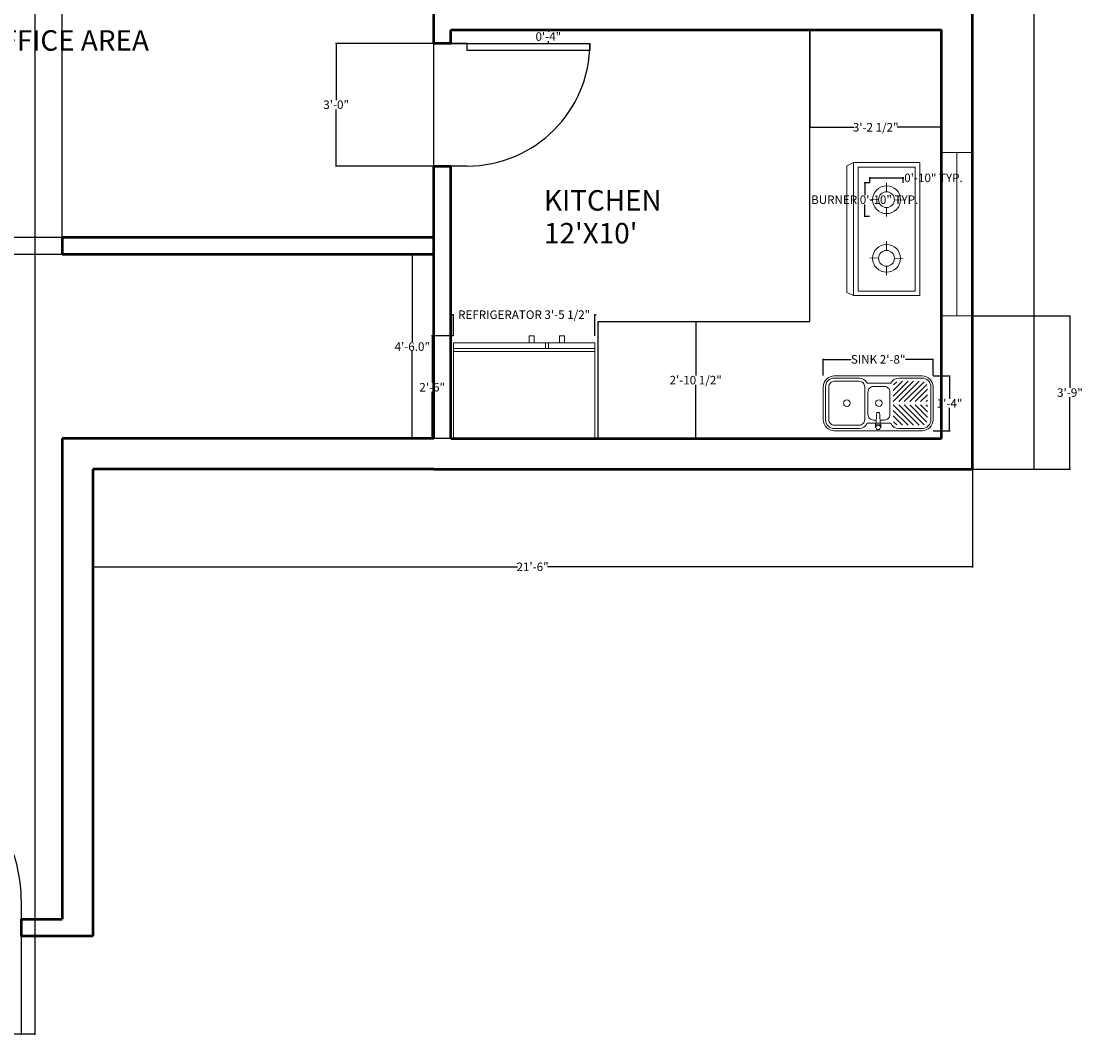
# Model space of a CAD drawing. Units: inches. Extents: x 9441 to 10027, y 18319 to 18830.
# Tile 3 of 4: x 9716 to 10027, y 18319 to 18618. Entities that reach past the tile are written whole.
import ezdxf

# ---------------------------------------------------------------- set-up
doc = ezdxf.new("R2010")
doc.units = ezdxf.units.IN
doc.header["$MEASUREMENT"] = 0
for name, color, linetype, lineweight in [('A-ANNO-DIMS', 2, 'Continuous', 18), ('A-AREA-IDEN', 7, 'Continuous', 25), ('A-DOOR', 3, 'Continuous', 25), ('A-FLOR-CABT', 9, 'Continuous', 25), ('A-FLOR-FIXT', 9, 'Continuous', 18), ('A-GLAZ', 4, 'Continuous', 18), ('A-WALL', 7, 'Continuous', 50), ('equipments', 8, 'Continuous', 20)]:
    doc.layers.add(name, color=color, linetype=linetype, lineweight=lineweight)
doc.styles.get("Standard").update_dxf_attribs({"font": 'arial.ttf'})
doc.dimstyles.get("Standard").update_dxf_attribs({"dimtxt": 2.5, "dimasz": 0.18, "dimexe": 0.18, "dimexo": 0.0625, "dimgap": 0.09, "dimtad": 0, "dimtih": 1, "dimtoh": 1, "dimdec": 1, "dimzin": 0, "dimdsep": 46, "dimlunit": 3, "dimtxsty": 'Standard', "dimcen": 0.09, "dimadec": 0, "dimazin": 0, "dimtfac": 1, "dimtdec": 1, "dimtofl": 0, "dimtmove": 0, "dimatfit": 3, "dimfxl": 1, "dimtolj": 1, "dimtzin": 0, "dimarcsym": 0})

# ---------------------------------------------------------------- blocks, each defined once
blk = doc.blocks.new('*U2')
for p, q in [((0, 0), (0, -100)), ((750, 0), (750, -100))]:
    blk.add_line(p, q)
blk.add_lwpolyline([(0, 0), (0, 750), (43.75, 750), (43.75, 0)], close=True)
blk.add_arc((0, 0), 750, 0, 90)
blk = doc.blocks.new('*U4')
for p, q in [((0, 100), (0, 0)), ((900, 100), (900, 0)), ((0, 50), (900, 50))]:
    blk.add_line(p, q)
blk = doc.blocks.new('C12')
for p, q in [((-0.70131, -0.87335), (-0.70131, -0.00485)), ((0.58127, -0.00485), (-0.70131, -0.00485)), ((0.58127, -0.87335), (0.58127, -0.00485)), ((-0.70131, -0.79423), (0.58127, -0.79423)), ((-0.70131, -0.82077), (0.58127, -0.82077)), ((-0.27938, -0.87335), (-0.27938, -0.82077)), ((-0.25493, -0.87335), (-0.25493, -0.82077)), ((-0.70131, -0.87335), (0.58127, -0.87335)), ((-0.42655, -0.93628), (-0.42655, -0.8713)), ((-0.38018, -0.8713), (-0.38018, -0.93628)), ((-0.15115, -0.8713), (-0.15115, -0.93628)), ((-0.10477, -0.93628), (-0.10477, -0.8713)), ((-0.38018, -0.93628), (-0.42655, -0.93628)), ((-0.15115, -0.93628), (-0.10477, -0.93628))]:
    blk.add_line(p, q)
blk = doc.blocks.new('62438789')
at = {"xscale": 10, "zscale": 10}
blk.add_blockref('C12', (0.9326, -0.0075), dxfattribs=at)
blk = doc.blocks.new('REFRIG4')
at = {"xscale": 0.1, "zscale": 0.1}
blk.add_blockref('62438789', (-0.0332, 0.0123), dxfattribs=at)
blk = doc.blocks.new('SINK_KITCHEN2')
for p, q in [((13.7, -23.5), (32.2, -5)), ((13.7, -13.5), (22.2, -5)), ((13.7, -18.5), (27.2, -5)), ((14.06, -8.14), (16.84, -5.36)), ((18.7, -23.5), (37.2, -5)), ((23.7, -23.5), (41.85, -5.35)), ((28.7, -23.5), (44.46, -7.74)), ((1.2, -16.49), (-1.2, -16.49)), ((33.7, -23.5), (45, -12.2)), ((38.7, -23.5), (45, -17.2)), ((13.7, -26.5), (32.2, -45)), ((18.7, -26.5), (37.2, -45)), ((23.7, -26.5), (41.85, -44.65)), ((28.7, -26.5), (44.46, -42.26)), ((33.7, -26.5), (45, -37.8)), ((38.7, -26.5), (45, -32.8)), ((43.7, -23.5), (45, -22.2)), ((43.7, -26.5), (45, -27.8)), ((13.7, -31.5), (27.2, -45)), ((13.7, -36.5), (22.2, -45)), ((14.06, -41.86), (16.84, -44.64))]:
    blk.add_line(p, q)
at = {"flags": 128}
for points in [[(-40, -50, -0.414214), (-50, -40), (-50, -10, -0.414214), (-40, 0), (40, 0, -0.414214), (50, -10), (50, -40, -0.414214), (40, -50)], [(-40, -45, -0.414214), (-45, -40), (-45, -10, -0.414214), (-40, -5), (-17.3, -5, -0.414214), (-12.3, -10), (-12.3, -40, -0.414214), (-17.3, -45)]]:
    blk.add_lwpolyline(points, format="xyb", close=True, dxfattribs=at)
for points in [[(2.5, -6.75), (11.39, -6.75, -0.296358), (18.7, -2), (40, -2, -0.414214), (48, -10), (48, -40, -0.414214), (40, -48), (18.7, -48, -0.296358), (11.39, -43.25), (-9.99, -43.25, -0.296358), (-17.3, -48), (-40, -48, -0.414214), (-48, -40), (-48, -10, -0.414214), (-40, -2), (-17.3, -2, -0.296358), (-9.99, -6.75), (-2.5, -6.75)], [(1.2, -16.49, 0.016708), (1.9, -6.98, 0.016708)], [(1.76, -9.75), (5.7, -9.75, -0.414214), (10.7, -14.75), (10.7, -35.25, -0.414214), (5.7, -40.25), (-4.3, -40.25, -0.414214), (-9.3, -35.25), (-9.3, -14.75, -0.414214), (-4.3, -9.75), (-1.76, -9.75)]]:
    blk.add_lwpolyline(points, format="xyb", dxfattribs=at)
blk.add_lwpolyline([(-2, -5.48), (2, -5.48), (2, -3), (2.5, -3), (2.5, -6.98), (-2.5, -6.98), (-2.5, -3), (-2, -3)], close=True)
for centre, radius in [((0, -3), 2), ((-28.65, -25), 3), ((0.7, -25), 3)]:
    blk.add_circle(centre, radius)
blk.add_arc((140.8, -1.2), 142.82, 182.31735, 186.14617)
blk = doc.blocks.new('*D14')
at = {"layer": 'A-ANNO-DIMS', "color": 0, "lineweight": -2, "transparency": 16777216}
for p, q in [((9836.83, 18549.93), (9830.42, 18549.93)), ((9830.6, 18549.75), (9830.6, 18524.29)), ((9830.6, 18496.11), (9830.6, 18521.56)), ((9836.83, 18495.93), (9830.42, 18495.93))]:
    blk.add_line(p, q, dxfattribs=at)
at = {"layer": 'A-ANNO-DIMS', "color": 0, "transparency": 16777216}
for points in [[(9830.57, 18549.75), (9830.63, 18549.75), (9830.6, 18549.93)], [(9830.57, 18496.11), (9830.63, 18496.11), (9830.6, 18495.93)]]:
    blk.add_solid(points, dxfattribs=at)
at = {"layer": 'Defpoints', "color": 0, "transparency": 16777216}
for p in [(9830.6, 18549.93), (9836.89, 18549.93), (9836.89, 18495.93)]:
    blk.add_point(p, dxfattribs=at)
at = {"layer": 'A-ANNO-DIMS', "color": 0, "transparency": 16777216, "insert": (9830.6, 18522.93), "char_height": 2.5, "attachment_point": 5}
blk.add_mtext('\\A1;4\'-6.0"', dxfattribs=at)
blk = doc.blocks.new('*D17')
at = {"layer": 'A-ANNO-DIMS', "color": 0, "lineweight": -2, "transparency": 16777216}
for p, q in [((9994.95, 18797.93), (10013.22, 18797.93)), ((10013.04, 18797.75), (10013.04, 18643.79)), ((10013.04, 18487.11), (10013.04, 18641.06)), ((9994.95, 18486.93), (10013.22, 18486.93))]:
    blk.add_line(p, q, dxfattribs=at)
at = {"layer": 'A-ANNO-DIMS', "color": 0, "transparency": 16777216}
for points in [[(10013.01, 18797.75), (10013.07, 18797.75), (10013.04, 18797.93)], [(10013.01, 18487.11), (10013.07, 18487.11), (10013.04, 18486.93)]]:
    blk.add_solid(points, dxfattribs=at)
at = {"layer": 'Defpoints', "color": 0, "transparency": 16777216}
for p in [(9994.89, 18797.93), (10013.04, 18797.93), (9994.89, 18486.93)]:
    blk.add_point(p, dxfattribs=at)
at = {"layer": 'A-ANNO-DIMS', "color": 0, "transparency": 16777216, "insert": (10013.04, 18642.43), "char_height": 2.5, "attachment_point": 5}
blk.add_mtext('\\A1;25\'-11.0"', dxfattribs=at)
blk = doc.blocks.new('WIN-FRAME-48x9')
for p, q in [((48, 9), (0, 9)), ((0, 9), (0, 0)), ((48, 0), (48, 9))]:
    blk.add_line(p, q)
blk = doc.blocks.new('COOKTOP-BURNER')
for p, q in [((4.94, 7.25), (4.95, 9.86)), ((2.61, 5), (0, 5.08)), ((7.25, 4.86), (9.85, 4.78)), ((4.92, 2.61), (4.9, 0))]:
    blk.add_line(p, q)
for radius in [4.08, 2.32]:
    blk.add_circle((4.93, 4.93), radius)
blk = doc.blocks.new('*D31')
at = {"layer": 'A-ANNO-DIMS', "color": 0, "lineweight": -2, "transparency": 16777216}
for p, q in [((9964.72, 18570.97), (9963.13, 18570.97)), ((9963.31, 18570.79), (9963.31, 18567.41)), ((9963.31, 18561.29), (9963.31, 18564.68)), ((9964.72, 18561.11), (9963.13, 18561.11))]:
    blk.add_line(p, q, dxfattribs=at)
at = {"layer": 'A-ANNO-DIMS', "color": 0, "transparency": 16777216}
for points in [[(9963.28, 18570.79), (9963.34, 18570.79), (9963.31, 18570.97)], [(9963.28, 18561.29), (9963.34, 18561.29), (9963.31, 18561.11)]]:
    blk.add_solid(points, dxfattribs=at)
at = {"layer": 'Defpoints', "color": 0, "transparency": 16777216}
for p in [(9963.31, 18570.97), (9964.79, 18570.97), (9964.79, 18561.11)]:
    blk.add_point(p, dxfattribs=at)
at = {"layer": 'A-ANNO-DIMS', "color": 0, "transparency": 16777216, "insert": (9963.31, 18566.04), "char_height": 2.5, "attachment_point": 5}
blk.add_mtext('\\A1;BURNER 0\'-10" TYP.', dxfattribs=at)
blk = doc.blocks.new('*D32')
at = {"layer": 'A-ANNO-DIMS', "color": 0, "lineweight": -2, "transparency": 16777216}
for p, q in [((9964.79, 18571.03), (9964.79, 18572.63)), ((9964.97, 18572.45), (9974.46, 18572.45)), ((9974.64, 18571.03), (9974.64, 18572.63)), ((9974.64, 18572.45), (9974.82, 18572.45))]:
    blk.add_line(p, q, dxfattribs=at)
at = {"layer": 'A-ANNO-DIMS', "color": 0, "transparency": 16777216}
for points in [[(9964.97, 18572.48), (9964.97, 18572.42), (9964.79, 18572.45)], [(9974.46, 18572.48), (9974.46, 18572.42), (9974.64, 18572.45)]]:
    blk.add_solid(points, dxfattribs=at)
at = {"layer": 'Defpoints', "color": 0, "transparency": 16777216}
for p in [(9974.64, 18572.45), (9964.79, 18570.97), (9974.64, 18570.97)]:
    blk.add_point(p, dxfattribs=at)
at = {"layer": 'A-ANNO-DIMS', "color": 0, "transparency": 16777216, "insert": (9983.5, 18572.45), "char_height": 2.5, "attachment_point": 5}
blk.add_mtext('\\A1;0\'-10" TYP.', dxfattribs=at)
blk = doc.blocks.new('*D33')
at = {"layer": 'A-ANNO-DIMS', "color": 0, "lineweight": -2, "transparency": 16777216}
for p, q in [((9842.49, 18532.3), (9842.31, 18532.3)), ((9842.67, 18526.13), (9842.67, 18532.48)), ((9884.18, 18526.13), (9884.18, 18532.48)), ((9884.36, 18532.3), (9884.54, 18532.3))]:
    blk.add_line(p, q, dxfattribs=at)
at = {"layer": 'A-ANNO-DIMS', "color": 0, "transparency": 16777216}
for points in [[(9842.49, 18532.33), (9842.49, 18532.27), (9842.67, 18532.3)], [(9884.36, 18532.33), (9884.36, 18532.27), (9884.18, 18532.3)]]:
    blk.add_solid(points, dxfattribs=at)
at = {"layer": 'Defpoints', "color": 0, "transparency": 16777216}
for p in [(9842.67, 18532.3), (9842.67, 18526.07), (9884.18, 18526.07)]:
    blk.add_point(p, dxfattribs=at)
at = {"layer": 'A-ANNO-DIMS', "color": 0, "transparency": 16777216, "insert": (9863.42, 18532.3), "char_height": 2.5, "attachment_point": 5}
blk.add_mtext('\\A1;REFRIGERATOR 3\'-5 1/2"', dxfattribs=at)
blk = doc.blocks.new('*D34')
at = {"layer": 'A-ANNO-DIMS', "color": 0, "lineweight": -2, "transparency": 16777216}
for p, q in [((9842.61, 18526.07), (9836.26, 18526.07)), ((9836.44, 18525.89), (9836.44, 18512.36)), ((9836.44, 18496.11), (9836.44, 18509.63)), ((9842.61, 18495.93), (9836.26, 18495.93))]:
    blk.add_line(p, q, dxfattribs=at)
at = {"layer": 'A-ANNO-DIMS', "color": 0, "transparency": 16777216}
for points in [[(9836.41, 18525.89), (9836.47, 18525.89), (9836.44, 18526.07)], [(9836.41, 18496.11), (9836.47, 18496.11), (9836.44, 18495.93)]]:
    blk.add_solid(points, dxfattribs=at)
at = {"layer": 'Defpoints', "color": 0, "transparency": 16777216}
for p in [(9842.67, 18526.07), (9836.44, 18495.93), (9842.67, 18495.93)]:
    blk.add_point(p, dxfattribs=at)
at = {"layer": 'A-ANNO-DIMS', "color": 0, "transparency": 16777216, "insert": (9836.44, 18511), "char_height": 2.5, "attachment_point": 5}
blk.add_mtext('\\A1;2\'-6"', dxfattribs=at)
blk = doc.blocks.new('*D35')
at = {"layer": 'A-ANNO-DIMS', "color": 0, "lineweight": -2, "transparency": 16777216}
for p, q in [((9951.17, 18514.41), (9951.17, 18519.36)), ((9951.35, 18519.18), (9959.3, 18519.18)), ((9983.19, 18519.18), (9975.24, 18519.18)), ((9983.37, 18514.41), (9983.37, 18519.36))]:
    blk.add_line(p, q, dxfattribs=at)
at = {"layer": 'A-ANNO-DIMS', "color": 0, "transparency": 16777216}
for points in [[(9951.35, 18519.21), (9951.35, 18519.15), (9951.17, 18519.18)], [(9983.19, 18519.21), (9983.19, 18519.15), (9983.37, 18519.18)]]:
    blk.add_solid(points, dxfattribs=at)
at = {"layer": 'Defpoints', "color": 0, "transparency": 16777216}
for p in [(9983.37, 18519.18), (9951.17, 18514.35), (9983.37, 18514.35)]:
    blk.add_point(p, dxfattribs=at)
at = {"layer": 'A-ANNO-DIMS', "color": 0, "transparency": 16777216, "insert": (9967.27, 18519.18), "char_height": 2.5, "attachment_point": 5}
blk.add_mtext('\\A1;SINK 2\'-8"', dxfattribs=at)
blk = doc.blocks.new('*D36')
at = {"layer": 'A-ANNO-DIMS', "color": 0, "lineweight": -2, "transparency": 16777216}
for p, q in [((9983.43, 18514.35), (9988.38, 18514.35)), ((9988.2, 18514.17), (9988.2, 18507.65)), ((9988.2, 18498.43), (9988.2, 18504.96)), ((9983.43, 18498.25), (9988.38, 18498.25))]:
    blk.add_line(p, q, dxfattribs=at)
at = {"layer": 'A-ANNO-DIMS', "color": 0, "transparency": 16777216}
for points in [[(9988.17, 18514.17), (9988.23, 18514.17), (9988.2, 18514.35)], [(9988.17, 18498.43), (9988.23, 18498.43), (9988.2, 18498.25)]]:
    blk.add_solid(points, dxfattribs=at)
at = {"layer": 'Defpoints', "color": 0, "transparency": 16777216}
for p in [(9983.37, 18514.35), (9983.37, 18498.25), (9988.2, 18498.25)]:
    blk.add_point(p, dxfattribs=at)
at = {"layer": 'A-ANNO-DIMS', "color": 0, "transparency": 16777216, "insert": (9988.2, 18506.3), "char_height": 2.5, "attachment_point": 5}
blk.add_mtext('\\A1;1\'-4"', dxfattribs=at)
blk = doc.blocks.new('*D37')
at = {"layer": 'A-ANNO-DIMS', "color": 0, "lineweight": -2, "transparency": 16777216}
for p, q in [((9736.89, 18486.86), (9736.89, 18458.12)), ((9994.89, 18486.86), (9994.89, 18458.12)), ((9737.07, 18458.3), (9861.49, 18458.3)), ((9994.71, 18458.3), (9870.3, 18458.3))]:
    blk.add_line(p, q, dxfattribs=at)
at = {"layer": 'A-ANNO-DIMS', "color": 0, "transparency": 16777216}
for points in [[(9737.07, 18458.33), (9737.07, 18458.27), (9736.89, 18458.3)], [(9994.71, 18458.33), (9994.71, 18458.27), (9994.89, 18458.3)]]:
    blk.add_solid(points, dxfattribs=at)
at = {"layer": 'Defpoints', "color": 0, "transparency": 16777216}
for p in [(9736.89, 18486.93), (9994.89, 18486.93), (9736.89, 18458.3)]:
    blk.add_point(p, dxfattribs=at)
at = {"layer": 'A-ANNO-DIMS', "color": 0, "transparency": 16777216, "insert": (9865.89, 18458.3), "char_height": 2.5, "attachment_point": 5}
blk.add_mtext('\\A1;21\'-6"', dxfattribs=at)
blk = doc.blocks.new('*D40')
at = {"layer": 'A-ANNO-DIMS', "color": 0, "lineweight": -2, "transparency": 16777216}
for p, q in [((9673.89, 18349.86), (9673.89, 18320.95)), ((9715.89, 18349.86), (9715.89, 18320.95)), ((9674.07, 18321.13), (9691.48, 18321.13)), ((9715.71, 18321.13), (9698.3, 18321.13))]:
    blk.add_line(p, q, dxfattribs=at)
at = {"layer": 'A-ANNO-DIMS', "color": 0, "transparency": 16777216}
for points in [[(9674.07, 18321.16), (9674.07, 18321.1), (9673.89, 18321.13)], [(9715.71, 18321.16), (9715.71, 18321.1), (9715.89, 18321.13)]]:
    blk.add_solid(points, dxfattribs=at)
at = {"layer": 'Defpoints', "color": 0, "transparency": 16777216}
for p in [(9673.89, 18349.93), (9715.89, 18349.93), (9715.89, 18321.13)]:
    blk.add_point(p, dxfattribs=at)
at = {"layer": 'A-ANNO-DIMS', "color": 0, "transparency": 16777216, "insert": (9694.89, 18321.13), "char_height": 2.5, "attachment_point": 5}
blk.add_mtext('\\A1;3\'-6"', dxfattribs=at)
blk = doc.blocks.new('*D46')
at = {"layer": 'A-ANNO-DIMS', "color": 0, "lineweight": -2, "transparency": 16777216}
for p, q in [((9994.95, 18531.93), (10023.7, 18531.93)), ((10023.52, 18531.75), (10023.52, 18510.79)), ((10023.52, 18487.11), (10023.52, 18508.06)), ((9994.95, 18486.93), (10023.7, 18486.93))]:
    blk.add_line(p, q, dxfattribs=at)
at = {"layer": 'A-ANNO-DIMS', "color": 0, "transparency": 16777216}
for points in [[(10023.49, 18531.75), (10023.55, 18531.75), (10023.52, 18531.93)], [(10023.49, 18487.11), (10023.55, 18487.11), (10023.52, 18486.93)]]:
    blk.add_solid(points, dxfattribs=at)
at = {"layer": 'Defpoints', "color": 0, "transparency": 16777216}
for p in [(9994.89, 18531.93), (10023.52, 18531.93), (9994.89, 18486.93)]:
    blk.add_point(p, dxfattribs=at)
at = {"layer": 'A-ANNO-DIMS', "color": 0, "transparency": 16777216, "insert": (10023.52, 18509.43), "char_height": 2.5, "attachment_point": 5}
blk.add_mtext('\\A1;3\'-9"', dxfattribs=at)
blk = doc.blocks.new('*D47')
at = {"layer": 'A-ANNO-DIMS', "color": 0, "lineweight": -2, "transparency": 16777216}
for p, q in [((9689.89, 18687.86), (9689.89, 18320.95)), ((9719.89, 18687.86), (9719.89, 18320.95)), ((9690.07, 18321.13), (9701.46, 18321.13)), ((9719.71, 18321.13), (9708.32, 18321.13))]:
    blk.add_line(p, q, dxfattribs=at)
at = {"layer": 'A-ANNO-DIMS', "color": 0, "transparency": 16777216}
for points in [[(9690.07, 18321.16), (9690.07, 18321.1), (9689.89, 18321.13)], [(9719.71, 18321.16), (9719.71, 18321.1), (9719.89, 18321.13)]]:
    blk.add_solid(points, dxfattribs=at)
at = {"layer": 'Defpoints', "color": 0, "transparency": 16777216}
for p in [(9689.89, 18687.93), (9719.89, 18687.93), (9719.89, 18321.13)]:
    blk.add_point(p, dxfattribs=at)
at = {"layer": 'A-ANNO-DIMS', "color": 0, "transparency": 16777216, "insert": (9704.89, 18321.13), "char_height": 2.5, "attachment_point": 5}
blk.add_mtext('\\A1;2\'-6"', dxfattribs=at)
blk = doc.blocks.new('*D53')
at = {"layer": 'A-ANNO-DIMS', "color": 0, "lineweight": -2, "transparency": 16777216}
for p, q in [((9836.83, 18611.93), (9808.09, 18611.93)), ((9808.27, 18611.75), (9808.27, 18595.29)), ((9808.27, 18576.11), (9808.27, 18592.56)), ((9836.83, 18575.93), (9808.09, 18575.93))]:
    blk.add_line(p, q, dxfattribs=at)
at = {"layer": 'A-ANNO-DIMS', "color": 0, "transparency": 16777216}
for points in [[(9808.24, 18611.75), (9808.3, 18611.75), (9808.27, 18611.93)], [(9808.24, 18576.11), (9808.3, 18576.11), (9808.27, 18575.93)]]:
    blk.add_solid(points, dxfattribs=at)
at = {"layer": 'Defpoints', "color": 0, "transparency": 16777216}
for p in [(9808.27, 18611.93), (9836.89, 18611.93), (9836.89, 18575.93)]:
    blk.add_point(p, dxfattribs=at)
at = {"layer": 'A-ANNO-DIMS', "color": 0, "transparency": 16777216, "insert": (9808.27, 18593.93), "char_height": 2.5, "attachment_point": 5}
blk.add_mtext('\\A1;3\'-0"', dxfattribs=at)
blk = doc.blocks.new('*D56')
at = {"layer": 'A-ANNO-DIMS', "color": 0, "lineweight": -2, "transparency": 16777216}
for p, q in [((9727.89, 18554.99), (9727.89, 18826.73)), ((9728.07, 18826.55), (9778.98, 18826.55)), ((9836.71, 18826.55), (9785.8, 18826.55)), ((9836.89, 18554.99), (9836.89, 18826.73))]:
    blk.add_line(p, q, dxfattribs=at)
at = {"layer": 'A-ANNO-DIMS', "color": 0, "transparency": 16777216}
for points in [[(9728.07, 18826.58), (9728.07, 18826.52), (9727.89, 18826.55)], [(9836.71, 18826.58), (9836.71, 18826.52), (9836.89, 18826.55)]]:
    blk.add_solid(points, dxfattribs=at)
at = {"layer": 'Defpoints', "color": 0, "transparency": 16777216}
for p in [(9836.89, 18826.55), (9727.89, 18554.93), (9836.89, 18554.93)]:
    blk.add_point(p, dxfattribs=at)
at = {"layer": 'A-ANNO-DIMS', "color": 0, "transparency": 16777216, "insert": (9782.39, 18826.55), "char_height": 2.5, "attachment_point": 5}
blk.add_mtext('\\A1;9\'-1"', dxfattribs=at)
blk = doc.blocks.new('*D57')
at = {"layer": 'A-ANNO-DIMS', "color": 0, "lineweight": -2, "transparency": 16777216}
for p, q in [((9727.83, 18554.93), (9699.09, 18554.93)), ((9699.27, 18554.75), (9699.27, 18553.79)), ((9727.83, 18549.93), (9699.09, 18549.93)), ((9699.27, 18550.11), (9699.27, 18551.06))]:
    blk.add_line(p, q, dxfattribs=at)
at = {"layer": 'A-ANNO-DIMS', "color": 0, "transparency": 16777216}
for points in [[(9699.24, 18554.75), (9699.3, 18554.75), (9699.27, 18554.93)], [(9699.24, 18550.11), (9699.3, 18550.11), (9699.27, 18549.93)]]:
    blk.add_solid(points, dxfattribs=at)
at = {"layer": 'Defpoints', "color": 0, "transparency": 16777216}
for p in [(9699.27, 18554.93), (9727.89, 18554.93), (9727.89, 18549.93)]:
    blk.add_point(p, dxfattribs=at)
at = {"layer": 'A-ANNO-DIMS', "color": 0, "transparency": 16777216, "insert": (9699.27, 18552.43), "char_height": 2.5, "attachment_point": 5}
blk.add_mtext('\\A1;0\'-5"', dxfattribs=at)
blk = doc.blocks.new('*D68')
at = {"layer": 'A-ANNO-DIMS', "color": 0, "lineweight": -2, "transparency": 16777216}
for p, q in [((9947.19, 18615.86), (9947.19, 18587.12)), ((9985.89, 18615.86), (9985.89, 18587.12)), ((9947.37, 18587.3), (9960.22, 18587.3)), ((9985.71, 18587.3), (9972.87, 18587.3))]:
    blk.add_line(p, q, dxfattribs=at)
at = {"layer": 'A-ANNO-DIMS', "color": 0, "transparency": 16777216}
for points in [[(9947.37, 18587.33), (9947.37, 18587.27), (9947.19, 18587.3)], [(9985.71, 18587.33), (9985.71, 18587.27), (9985.89, 18587.3)]]:
    blk.add_solid(points, dxfattribs=at)
at = {"layer": 'Defpoints', "color": 0, "transparency": 16777216}
for p in [(9947.19, 18615.93), (9985.89, 18615.93), (9947.19, 18587.3)]:
    blk.add_point(p, dxfattribs=at)
at = {"layer": 'A-ANNO-DIMS', "color": 0, "transparency": 16777216, "insert": (9966.54, 18587.3), "char_height": 2.5, "attachment_point": 5}
blk.add_mtext('\\A1;3\'-2 1/2"', dxfattribs=at)
blk = doc.blocks.new('*D69')
at = {"layer": 'A-ANNO-DIMS', "color": 0, "lineweight": -2, "transparency": 16777216}
for p, q in [((9885.17, 18530.25), (9913.91, 18530.25)), ((9913.73, 18530.07), (9913.73, 18514.47)), ((9913.73, 18496.11), (9913.73, 18511.71)), ((9885.17, 18495.93), (9913.91, 18495.93))]:
    blk.add_line(p, q, dxfattribs=at)
at = {"layer": 'A-ANNO-DIMS', "color": 0, "transparency": 16777216}
for points in [[(9913.7, 18530.07), (9913.76, 18530.07), (9913.73, 18530.25)], [(9913.7, 18496.11), (9913.76, 18496.11), (9913.73, 18495.93)]]:
    blk.add_solid(points, dxfattribs=at)
at = {"layer": 'Defpoints', "color": 0, "transparency": 16777216}
for p in [(9885.11, 18530.25), (9885.11, 18495.93), (9913.73, 18495.93)]:
    blk.add_point(p, dxfattribs=at)
at = {"layer": 'A-ANNO-DIMS', "color": 0, "transparency": 16777216, "insert": (9913.73, 18513.09), "char_height": 2.5, "attachment_point": 5}
blk.add_mtext('\\A1;2\'-10 1/2"', dxfattribs=at)
blk = doc.blocks.new('*D73')
at = {"layer": 'A-ANNO-DIMS', "color": 0, "lineweight": -2, "transparency": 16777216}
for p, q in [((9841.95, 18615.93), (9870.7, 18615.93)), ((9870.52, 18615.75), (9870.52, 18615.29)), ((9841.95, 18611.93), (9870.7, 18611.93)), ((9870.52, 18612.11), (9870.52, 18612.56))]:
    blk.add_line(p, q, dxfattribs=at)
at = {"layer": 'A-ANNO-DIMS', "color": 0, "transparency": 16777216}
for points in [[(9870.49, 18615.75), (9870.55, 18615.75), (9870.52, 18615.93)], [(9870.49, 18612.11), (9870.55, 18612.11), (9870.52, 18611.93)]]:
    blk.add_solid(points, dxfattribs=at)
at = {"layer": 'Defpoints', "color": 0, "transparency": 16777216}
for p in [(9841.89, 18615.93), (9841.89, 18611.93), (9870.52, 18611.93)]:
    blk.add_point(p, dxfattribs=at)
at = {"layer": 'A-ANNO-DIMS', "color": 0, "transparency": 16777216, "insert": (9870.52, 18613.93), "char_height": 2.5, "attachment_point": 5}
blk.add_mtext('\\A1;0\'-4"', dxfattribs=at)

msp = doc.modelspace()

# ---------------------------------------------------------------- linework, layer by layer
at = {"layer": 'A-FLOR-CABT'}
for p, q in [((9947.19, 18530.25), (9947.19, 18615.93)), ((9885.11, 18530.25), (9947.19, 18530.25)), ((9885.11, 18495.93), (9885.11, 18530.25))]:
    msp.add_line(p, q, dxfattribs=at)
at = {"layer": 'A-WALL'}
for p, q in [((9994.89, 18486.93), (9994.89, 18797.93)), ((9836.89, 18611.93), (9836.89, 18624.93)), ((9841.89, 18615.93), (9985.89, 18615.93)), ((9841.89, 18611.93), (9841.89, 18615.93)), ((9985.89, 18495.93), (9985.89, 18615.93)), ((9841.89, 18611.93), (9836.89, 18611.93)), ((9836.89, 18495.93), (9836.89, 18575.93)), ((9836.89, 18575.93), (9841.89, 18575.93)), ((9841.89, 18495.93), (9841.89, 18575.93)), ((9836.89, 18554.93), (9727.89, 18554.93)), ((9727.89, 18554.93), (9727.89, 18549.93)), ((9836.89, 18549.93), (9727.89, 18549.93)), ((9727.89, 18495.93), (9727.89, 18354.93)), ((9836.89, 18495.93), (9727.89, 18495.93)), ((9841.89, 18495.93), (9985.89, 18495.93)), ((9836.89, 18486.93), (9736.89, 18486.93)), ((9736.89, 18486.93), (9736.89, 18349.93)), ((9836.89, 18486.93), (9994.89, 18486.93)), ((9715.89, 18354.93), (9715.89, 18349.93)), ((9715.89, 18354.93), (9727.89, 18354.93)), ((9736.89, 18349.93), (9715.89, 18349.93))]:
    msp.add_line(p, q, dxfattribs=at)
at = {"layer": 'equipments'}
for p, q in [((9960.07, 18576.92), (9958.09, 18576.01)), ((9958.09, 18576.01), (9958.09, 18538.79)), ((9979.46, 18576.92), (9960.07, 18576.92)), ((9960.07, 18576.92), (9960.07, 18537.88)), ((9978.16, 18575.61), (9961.38, 18575.61)), ((9961.38, 18575.61), (9961.38, 18539.19)), ((9978.16, 18575.61), (9978.16, 18539.19)), ((9979.46, 18576.92), (9979.46, 18537.88)), ((9960.07, 18537.88), (9958.09, 18538.79)), ((9979.46, 18537.88), (9960.07, 18537.88)), ((9978.16, 18539.19), (9961.38, 18539.19))]:
    msp.add_line(p, q, dxfattribs=at)

# ---------------------------------------------------------------- block references
at = {"layer": 'A-DOOR', "xscale": 0.0480000000000006, "yscale": 0.0480000000000006, "zscale": 0.0480000000000006, "rotation": 270}
msp.add_blockref('*U2', (9846.69, 18611.93), dxfattribs=at)
at = {"layer": 'A-DOOR', "xscale": 0.0560000000000007, "yscale": 0.0560000000000007, "zscale": 0.0560000000000007}
msp.add_blockref('*U2', (9673.89, 18360.53), dxfattribs=at)
at = {"layer": 'A-FLOR-FIXT', "xscale": -0.3219716873091472, "yscale": 0.3219716873091472, "zscale": 0.3219716873091472, "rotation": 180}
msp.add_blockref('SINK_KITCHEN2', (9967.27, 18498.25), dxfattribs=at)
at = {"layer": 'A-GLAZ', "rotation": 269.999999999999}
msp.add_blockref('WIN-FRAME-48x9', (9985.89, 18579.93), dxfattribs=at)
at = {"layer": 'A-GLAZ', "xscale": 0.0533333333333332, "yscale": 0.0533333333333332, "zscale": 0.0533333333333332, "rotation": 270}
msp.add_blockref('*U4', (9987.72, 18579.93), dxfattribs=at)
at = {"layer": 'equipments'}
msp.add_blockref('COOKTOP-BURNER', (9964.79, 18561.11), dxfattribs=at)
at = {"layer": 'equipments', "rotation": 180}
msp.add_blockref('COOKTOP-BURNER', (9974.64, 18553.77), dxfattribs=at)
at = {"layer": 'equipments', "xscale": 32.36273076194324, "yscale": 32.36273076194324, "zscale": 32.36273076194324, "rotation": 180}
msp.add_blockref('REFRIG4', (9863.42, 18495.93), dxfattribs=at)

# ---------------------------------------------------------------- texts
at = {"layer": 'A-AREA-IDEN'}
for s, p in [('OPEN OFFICE AREA', (9680.17, 18609.79)), ('KITCHEN', (9869.24, 18562.85)), ("12'X10'", (9869.24, 18553.21))]:
    msp.add_text(s, height=6, dxfattribs=at).set_placement(p)

# ---------------------------------------------------------------- dimensions: what is measured, and where the dimension line sits
at = {"layer": 'A-ANNO-DIMS'}
for base, p1, p2, picture, middle in [((9836.89, 18826.55), (9727.89, 18554.93), (9836.89, 18554.93), '*D56', (9782.39, 18826.55)), ((9719.89, 18321.13), (9689.89, 18687.93), (9719.89, 18687.93), '*D47', (9704.89, 18321.13)), ((9715.89, 18321.13), (9673.89, 18349.93), (9715.89, 18349.93), '*D40', (9694.89, 18321.13))]:
    dim = msp.add_linear_dim(base=base, p1=p1, p2=p2, dimstyle='Standard', override={"dimdec": 1, "dimlfac": 1, "dimrnd": 0, "dimzin": 1, "dimdsep": 46, "dimlunit": 4, "dimfrac": 2}, dxfattribs=at)
    dim.commit()
    dim.dimension.update_dxf_attribs({"geometry": picture, "text_midpoint": middle})
for base, p1, p2, angle, override, picture, middle in [((10013.04, 18797.93), (9994.89, 18486.93), (9994.89, 18797.93), 90, {"dimclrd": 0, "dimclre": 0, "dimclrt": 0}, '*D17', (10013.04, 18642.43)), ((9870.52, 18611.93), (9841.89, 18615.93), (9841.89, 18611.93), 270, {"dimdec": 1, "dimlfac": 1, "dimrnd": 0, "dimzin": 1, "dimdsep": 46, "dimlunit": 4, "dimfrac": 2}, '*D73', (9870.52, 18613.93)), ((9947.19, 18587.3), (9985.89, 18615.93), (9947.19, 18615.93), 180, {"dimdec": 1, "dimlfac": 1, "dimrnd": 0, "dimzin": 1, "dimdsep": 46, "dimlunit": 4, "dimfrac": 2}, '*D68', (9966.54, 18587.3)), ((9808.27, 18611.93), (9836.89, 18575.93), (9836.89, 18611.93), 90, {"dimdec": 1, "dimlfac": 1, "dimrnd": 0, "dimzin": 1, "dimdsep": 46, "dimlunit": 4, "dimfrac": 2}, '*D53', (9808.27, 18593.93)), ((9699.27, 18554.93), (9727.89, 18549.93), (9727.89, 18554.93), 90, {"dimdec": 1, "dimlfac": 1, "dimrnd": 0, "dimzin": 1, "dimdsep": 46, "dimlunit": 4, "dimfrac": 2}, '*D57', (9699.27, 18552.43)), ((9830.6, 18549.93), (9836.89, 18495.93), (9836.89, 18549.93), 90, {"dimclrd": 0, "dimclre": 0, "dimclrt": 0}, '*D14', (9830.6, 18522.93)), ((10023.52, 18531.93), (9994.89, 18486.93), (9994.89, 18531.93), 90, {"dimdec": 1, "dimlfac": 1, "dimrnd": 0, "dimzin": 1, "dimdsep": 46, "dimlunit": 4, "dimfrac": 2}, '*D46', (10023.52, 18509.43)), ((9913.73, 18495.93), (9885.11, 18530.25), (9885.11, 18495.93), 270, {"dimdec": 1, "dimlfac": 1, "dimrnd": 0, "dimzin": 1, "dimdsep": 46, "dimlunit": 4, "dimfrac": 2}, '*D69', (9913.73, 18513.09)), ((9836.44, 18495.93), (9842.67, 18526.07), (9842.67, 18495.93), 270, {"dimdec": 1, "dimlfac": 1, "dimrnd": 0, "dimzin": 1, "dimdsep": 46, "dimlunit": 4, "dimfrac": 2}, '*D34', (9836.44, 18511)), ((9988.2, 18498.25), (9983.37, 18514.35), (9983.37, 18498.25), 270, {"dimdec": 1, "dimlfac": 1, "dimrnd": 0, "dimzin": 1, "dimdsep": 46, "dimlunit": 4, "dimfrac": 2}, '*D36', (9988.2, 18506.3)), ((9736.89, 18458.3), (9994.89, 18486.93), (9736.89, 18486.93), 180, {"dimdec": 1, "dimlfac": 1, "dimrnd": 0, "dimzin": 1, "dimdsep": 46, "dimlunit": 4, "dimfrac": 2}, '*D37', (9865.89, 18458.3))]:
    dim = msp.add_linear_dim(base=base, p1=p1, p2=p2, angle=angle, dimstyle='Standard', override=override, dxfattribs=at)
    dim.commit()
    dim.dimension.update_dxf_attribs({"geometry": picture, "text_midpoint": middle})
for base, p1, p2, text, picture, middle in [((9974.6406, 18572.4512), (9964.7862, 18570.9723), (9974.6406, 18570.9723), '<> TYP.', '*D32', (9983.5012, 18572.4512)), ((9983.37, 18519.18), (9951.17, 18514.35), (9983.37, 18514.35), 'SINK <>', '*D35', (9967.27, 18519.18))]:
    dim = msp.add_linear_dim(base=base, p1=p1, p2=p2, text=text, dimstyle='Standard', override={"dimdec": 1, "dimlfac": 1, "dimrnd": 0, "dimzin": 1, "dimdsep": 46, "dimlunit": 4, "dimfrac": 2}, dxfattribs=at)
    dim.commit()
    dim.dimension.update_dxf_attribs({"geometry": picture, "text_midpoint": middle})
for base, p1, p2, angle, text, picture, middle in [((9963.31, 18570.97), (9964.79, 18561.11), (9964.79, 18570.97), 90, 'BURNER <> TYP.', '*D31', (9963.31, 18566.04)), ((9842.67, 18532.3), (9884.18, 18526.07), (9842.67, 18526.07), 180, 'REFRIGERATOR <>', '*D33', (9863.42, 18532.3))]:
    dim = msp.add_linear_dim(base=base, p1=p1, p2=p2, angle=angle, text=text, dimstyle='Standard', override={"dimdec": 1, "dimlfac": 1, "dimrnd": 0, "dimzin": 1, "dimdsep": 46, "dimlunit": 4, "dimfrac": 2}, dxfattribs=at)
    dim.commit()
    dim.dimension.update_dxf_attribs({"geometry": picture, "text_midpoint": middle})

doc.saveas('drawing.dxf')
